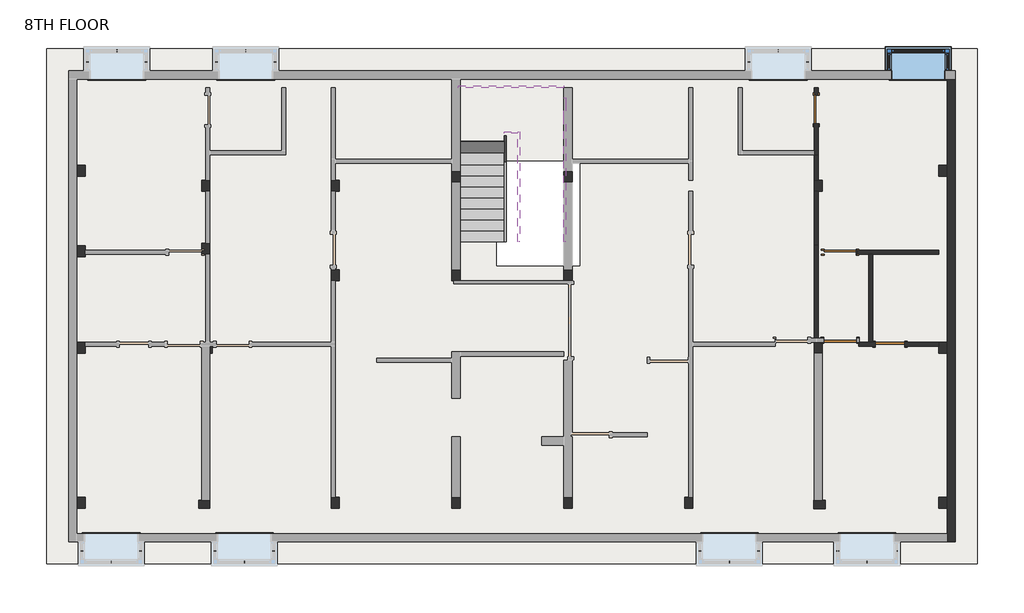
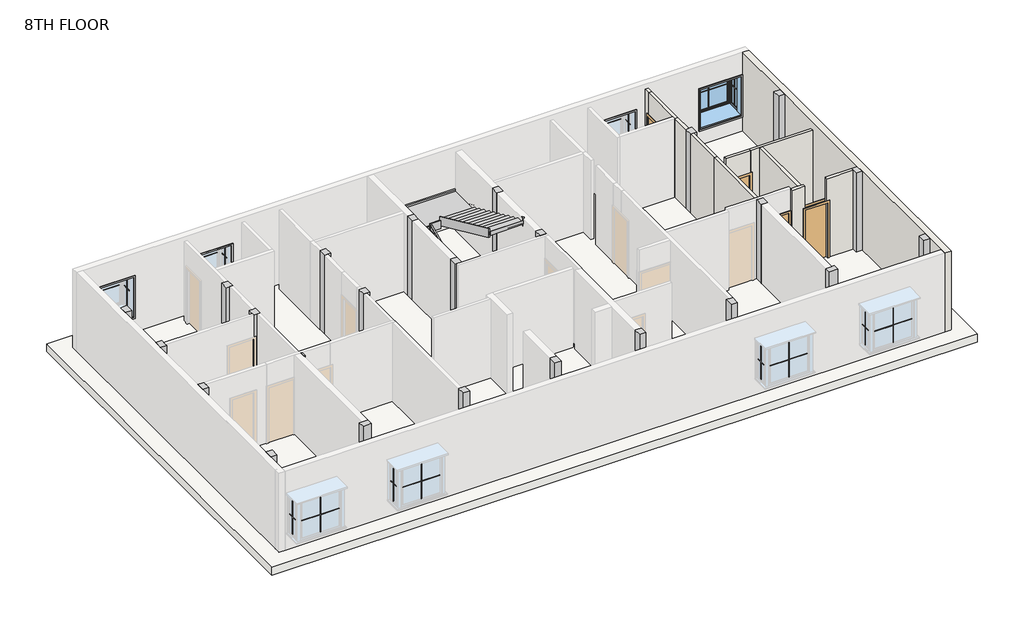
# One storey, part 2 of 2: 32 proxies, 24 columns, 11 walls, 6 members, 4 doors, 1 slab, 1 stair flight, 1 window.
"""IFC4 building model written with IfcOpenShell, lengths in millimetres."""

from ifc_helpers import new_model, si_unit, frame, origin, place, context, project, spatial, polyline, outline, extrude, faceted_brep, transform, mapped, element, save
from components import m_muntin_pattern_2x2_m_muntin_pattern_2x2_c1fd4460, m_muntin_pattern_2x2_m_muntin_pattern_2x2_777b163a, m_trim_window_interior_flat_picture_frame_44e8afef, column_68c8e778, door_1991e9a2, door_a431d384, door_82def9da, m_door_single_panel_3_x7_f8176753, stair_flight_66ca282f, window_19bbd869

model = new_model("IFC4")

# Units and contexts
model_context = context("Model", 3, world=origin())
ifc_project = project(units=[si_unit("LENGTHUNIT", "METRE", prefix="MILLI")], contexts=[model_context])

# Site, building, storey
site = spatial("IfcSite", under=ifc_project)
building = spatial("IfcBuilding", under=site)
storey = spatial("IfcBuildingStorey", under=building, Name="8TH FLOOR", Elevation=28803.6)

# Proxies
placement = place(None, origin())
m_muntin_pattern_2x2_m_muntin_pattern_2x2_shape = m_muntin_pattern_2x2_m_muntin_pattern_2x2_c1fd4460(model_context)
element("IfcBuildingElementProxy", 1, Name="M_Muntin Pattern_2x2 : M_Muntin Pattern_2x2", ObjectType="M_Muntin Pattern_2x2 : M_Muntin Pattern_2x2", at=placement, inside=storey, context=model_context, shape_type="MappedRepresentation", body=[
    mapped(m_muntin_pattern_2x2_m_muntin_pattern_2x2_shape, transform((-11500.7987957, -5499.9182661, 29524.25), x_axis=(-1.0, 0.0, 0.0), y_axis=(0.0, -1.0, 0.0), z_axis=(0.0, 0.0, 1.0))),
])
element("IfcBuildingElementProxy", 2, Name="M_Muntin Pattern_2x2 : M_Muntin Pattern_2x2", ObjectType="M_Muntin Pattern_2x2 : M_Muntin Pattern_2x2", at=placement, inside=storey, context=model_context, shape_type="MappedRepresentation", body=[
    mapped(m_muntin_pattern_2x2_m_muntin_pattern_2x2_shape, transform((-7819.250543, -5499.9182661, 29524.25), x_axis=(-1.0, 0.0, 0.0), y_axis=(0.0, -1.0, 0.0), z_axis=(0.0, 0.0, 1.0))),
])
element("IfcBuildingElementProxy", 3, Name="M_Muntin Pattern_2x2 : M_Muntin Pattern_2x2", ObjectType="M_Muntin Pattern_2x2 : M_Muntin Pattern_2x2", at=placement, inside=storey, context=model_context, shape_type="MappedRepresentation", body=[
    mapped(m_muntin_pattern_2x2_m_muntin_pattern_2x2_shape, transform((5599.7512082, -5499.9182661, 29524.25), x_axis=(-1.0, 0.0, 0.0), y_axis=(0.0, -1.0, 0.0), z_axis=(0.0, 0.0, 1.0))),
])
element("IfcBuildingElementProxy", 4, Name="M_Muntin Pattern_2x2 : M_Muntin Pattern_2x2", ObjectType="M_Muntin Pattern_2x2 : M_Muntin Pattern_2x2", at=placement, inside=storey, context=model_context, shape_type="MappedRepresentation", body=[
    mapped(m_muntin_pattern_2x2_m_muntin_pattern_2x2_shape, transform((9408.6146942, -5499.9182662, 29524.25), x_axis=(-1.0, 0.0, 0.0), y_axis=(0.0, -1.0, 0.0), z_axis=(0.0, 0.0, 1.0))),
])
element("IfcBuildingElementProxy", 5, Name="M_Muntin Pattern_2x2 : M_Muntin Pattern_2x2", ObjectType="M_Muntin Pattern_2x2 : M_Muntin Pattern_2x2", at=placement, inside=storey, context=model_context, shape_type="MappedRepresentation", body=[
    mapped(m_muntin_pattern_2x2_m_muntin_pattern_2x2_shape, transform((-11348.3987957, 8647.7317329, 29524.25), x_axis=(1.0, 0.0, 0.0), y_axis=(0.0, 1.0, 0.0), z_axis=(0.0, 0.0, 1.0))),
])
element("IfcBuildingElementProxy", 6, Name="M_Muntin Pattern_2x2 : M_Muntin Pattern_2x2", ObjectType="M_Muntin Pattern_2x2 : M_Muntin Pattern_2x2", at=placement, inside=storey, context=model_context, shape_type="MappedRepresentation", body=[
    mapped(m_muntin_pattern_2x2_m_muntin_pattern_2x2_shape, transform((-7779.6987993, 8647.7317329, 29524.25), x_axis=(1.0, 0.0, 0.0), y_axis=(0.0, 1.0, 0.0), z_axis=(0.0, 0.0, 1.0))),
])
element("IfcBuildingElementProxy", 7, Name="M_Muntin Pattern_2x2 : M_Muntin Pattern_2x2", ObjectType="M_Muntin Pattern_2x2 : M_Muntin Pattern_2x2", at=placement, inside=storey, context=model_context, shape_type="MappedRepresentation", body=[
    mapped(m_muntin_pattern_2x2_m_muntin_pattern_2x2_shape, transform((6952.301208, 8647.7317329, 29524.25), x_axis=(1.0, 0.0, 0.0), y_axis=(0.0, 1.0, 0.0), z_axis=(0.0, 0.0, 1.0))),
])
element("IfcBuildingElementProxy", 8, Name="M_Muntin Pattern_2x2 : M_Muntin Pattern_2x2", ObjectType="M_Muntin Pattern_2x2 : M_Muntin Pattern_2x2", at=placement, inside=storey, context=model_context, shape_type="MappedRepresentation", body=[
    mapped(m_muntin_pattern_2x2_m_muntin_pattern_2x2_shape, transform((10825.8012075, 8647.7317329, 29524.25), x_axis=(1.0, 0.0, 0.0), y_axis=(0.0, 1.0, 0.0), z_axis=(0.0, 0.0, 1.0))),
])
m_muntin_pattern_2x2_m_muntin_pattern_2x2_2_shape = m_muntin_pattern_2x2_m_muntin_pattern_2x2_777b163a(model_context)
element("IfcBuildingElementProxy", 9, Name="M_Muntin Pattern_2x2 : M_Muntin Pattern_2x2", ObjectType="M_Muntin Pattern_2x2 : M_Muntin Pattern_2x2", at=placement, inside=storey, context=model_context, shape_type="MappedRepresentation", body=[
    mapped(m_muntin_pattern_2x2_m_muntin_pattern_2x2_2_shape, transform((-10690.4737957, -5190.3932661, 29524.25), x_axis=(0.0, 1.0, 0.0), y_axis=(-1.0, 0.0, 0.0), z_axis=(0.0, 0.0, 1.0))),
])
element("IfcBuildingElementProxy", 10, Name="M_Muntin Pattern_2x2 : M_Muntin Pattern_2x2", ObjectType="M_Muntin Pattern_2x2 : M_Muntin Pattern_2x2", at=placement, inside=storey, context=model_context, shape_type="MappedRepresentation", body=[
    mapped(m_muntin_pattern_2x2_m_muntin_pattern_2x2_2_shape, transform((-12311.1237957, -5190.3932661, 29524.25), x_axis=(0.0, -1.0, 0.0), y_axis=(1.0, 0.0, 0.0), z_axis=(0.0, 0.0, 1.0))),
])
element("IfcBuildingElementProxy", 11, Name="M_Muntin Pattern_2x2 : M_Muntin Pattern_2x2", ObjectType="M_Muntin Pattern_2x2 : M_Muntin Pattern_2x2", at=placement, inside=storey, context=model_context, shape_type="MappedRepresentation", body=[
    mapped(m_muntin_pattern_2x2_m_muntin_pattern_2x2_2_shape, transform((-7008.925543, -5190.3932661, 29524.25), x_axis=(0.0, 1.0, 0.0), y_axis=(-1.0, 0.0, 0.0), z_axis=(0.0, 0.0, 1.0))),
])
element("IfcBuildingElementProxy", 12, Name="M_Muntin Pattern_2x2 : M_Muntin Pattern_2x2", ObjectType="M_Muntin Pattern_2x2 : M_Muntin Pattern_2x2", at=placement, inside=storey, context=model_context, shape_type="MappedRepresentation", body=[
    mapped(m_muntin_pattern_2x2_m_muntin_pattern_2x2_2_shape, transform((-8629.575543, -5190.3932661, 29524.25), x_axis=(0.0, -1.0, 0.0), y_axis=(1.0, 0.0, 0.0), z_axis=(0.0, 0.0, 1.0))),
])
element("IfcBuildingElementProxy", 13, Name="M_Muntin Pattern_2x2 : M_Muntin Pattern_2x2", ObjectType="M_Muntin Pattern_2x2 : M_Muntin Pattern_2x2", at=placement, inside=storey, context=model_context, shape_type="MappedRepresentation", body=[
    mapped(m_muntin_pattern_2x2_m_muntin_pattern_2x2_2_shape, transform((6410.0762082, -5190.3932661, 29524.25), x_axis=(0.0, 1.0, 0.0), y_axis=(-1.0, 0.0, 0.0), z_axis=(0.0, 0.0, 1.0))),
])
element("IfcBuildingElementProxy", 14, Name="M_Muntin Pattern_2x2 : M_Muntin Pattern_2x2", ObjectType="M_Muntin Pattern_2x2 : M_Muntin Pattern_2x2", at=placement, inside=storey, context=model_context, shape_type="MappedRepresentation", body=[
    mapped(m_muntin_pattern_2x2_m_muntin_pattern_2x2_2_shape, transform((4789.4262082, -5190.3932661, 29524.25), x_axis=(0.0, -1.0, 0.0), y_axis=(1.0, 0.0, 0.0), z_axis=(0.0, 0.0, 1.0))),
])
element("IfcBuildingElementProxy", 15, Name="M_Muntin Pattern_2x2 : M_Muntin Pattern_2x2", ObjectType="M_Muntin Pattern_2x2 : M_Muntin Pattern_2x2", at=placement, inside=storey, context=model_context, shape_type="MappedRepresentation", body=[
    mapped(m_muntin_pattern_2x2_m_muntin_pattern_2x2_2_shape, transform((10218.9396942, -5190.3932662, 29524.25), x_axis=(0.0, 1.0, 0.0), y_axis=(-1.0, 0.0, 0.0), z_axis=(0.0, 0.0, 1.0))),
])
element("IfcBuildingElementProxy", 16, Name="M_Muntin Pattern_2x2 : M_Muntin Pattern_2x2", ObjectType="M_Muntin Pattern_2x2 : M_Muntin Pattern_2x2", at=placement, inside=storey, context=model_context, shape_type="MappedRepresentation", body=[
    mapped(m_muntin_pattern_2x2_m_muntin_pattern_2x2_2_shape, transform((8598.2896942, -5190.3932661, 29524.25), x_axis=(0.0, -1.0, 0.0), y_axis=(1.0, 0.0, 0.0), z_axis=(0.0, 0.0, 1.0))),
])
element("IfcBuildingElementProxy", 17, Name="M_Muntin Pattern_2x2 : M_Muntin Pattern_2x2", ObjectType="M_Muntin Pattern_2x2 : M_Muntin Pattern_2x2", at=placement, inside=storey, context=model_context, shape_type="MappedRepresentation", body=[
    mapped(m_muntin_pattern_2x2_m_muntin_pattern_2x2_2_shape, transform((-12158.7237957, 8338.2067329, 29524.25), x_axis=(0.0, -1.0, 0.0), y_axis=(1.0, 0.0, 0.0), z_axis=(0.0, 0.0, 1.0))),
])
element("IfcBuildingElementProxy", 18, Name="M_Muntin Pattern_2x2 : M_Muntin Pattern_2x2", ObjectType="M_Muntin Pattern_2x2 : M_Muntin Pattern_2x2", at=placement, inside=storey, context=model_context, shape_type="MappedRepresentation", body=[
    mapped(m_muntin_pattern_2x2_m_muntin_pattern_2x2_2_shape, transform((-10538.0737957, 8338.2067329, 29524.25), x_axis=(0.0, 1.0, 0.0), y_axis=(-1.0, 0.0, 0.0), z_axis=(0.0, 0.0, 1.0))),
])
element("IfcBuildingElementProxy", 19, Name="M_Muntin Pattern_2x2 : M_Muntin Pattern_2x2", ObjectType="M_Muntin Pattern_2x2 : M_Muntin Pattern_2x2", at=placement, inside=storey, context=model_context, shape_type="MappedRepresentation", body=[
    mapped(m_muntin_pattern_2x2_m_muntin_pattern_2x2_2_shape, transform((-8590.0237993, 8338.2067329, 29524.25), x_axis=(0.0, -1.0, 0.0), y_axis=(1.0, 0.0, 0.0), z_axis=(0.0, 0.0, 1.0))),
])
element("IfcBuildingElementProxy", 20, Name="M_Muntin Pattern_2x2 : M_Muntin Pattern_2x2", ObjectType="M_Muntin Pattern_2x2 : M_Muntin Pattern_2x2", at=placement, inside=storey, context=model_context, shape_type="MappedRepresentation", body=[
    mapped(m_muntin_pattern_2x2_m_muntin_pattern_2x2_2_shape, transform((-6969.3737993, 8338.2067329, 29524.25), x_axis=(0.0, 1.0, 0.0), y_axis=(-1.0, 0.0, 0.0), z_axis=(0.0, 0.0, 1.0))),
])
element("IfcBuildingElementProxy", 21, Name="M_Muntin Pattern_2x2 : M_Muntin Pattern_2x2", ObjectType="M_Muntin Pattern_2x2 : M_Muntin Pattern_2x2", at=placement, inside=storey, context=model_context, shape_type="MappedRepresentation", body=[
    mapped(m_muntin_pattern_2x2_m_muntin_pattern_2x2_2_shape, transform((6141.976208, 8338.2067329, 29524.25), x_axis=(0.0, -1.0, 0.0), y_axis=(1.0, 0.0, 0.0), z_axis=(0.0, 0.0, 1.0))),
])
element("IfcBuildingElementProxy", 22, Name="M_Muntin Pattern_2x2 : M_Muntin Pattern_2x2", ObjectType="M_Muntin Pattern_2x2 : M_Muntin Pattern_2x2", at=placement, inside=storey, context=model_context, shape_type="MappedRepresentation", body=[
    mapped(m_muntin_pattern_2x2_m_muntin_pattern_2x2_2_shape, transform((7762.626208, 8338.2067329, 29524.25), x_axis=(0.0, 1.0, 0.0), y_axis=(-1.0, 0.0, 0.0), z_axis=(0.0, 0.0, 1.0))),
])
element("IfcBuildingElementProxy", 23, Name="M_Muntin Pattern_2x2 : M_Muntin Pattern_2x2", ObjectType="M_Muntin Pattern_2x2 : M_Muntin Pattern_2x2", at=placement, inside=storey, context=model_context, shape_type="MappedRepresentation", body=[
    mapped(m_muntin_pattern_2x2_m_muntin_pattern_2x2_2_shape, transform((10015.4762075, 8338.2067329, 29524.25), x_axis=(0.0, -1.0, 0.0), y_axis=(1.0, 0.0, 0.0), z_axis=(0.0, 0.0, 1.0))),
])
element("IfcBuildingElementProxy", 24, Name="M_Muntin Pattern_2x2 : M_Muntin Pattern_2x2", ObjectType="M_Muntin Pattern_2x2 : M_Muntin Pattern_2x2", at=placement, inside=storey, context=model_context, shape_type="MappedRepresentation", body=[
    mapped(m_muntin_pattern_2x2_m_muntin_pattern_2x2_2_shape, transform((11636.1262075, 8338.2067329, 29524.25), x_axis=(0.0, 1.0, 0.0), y_axis=(-1.0, 0.0, 0.0), z_axis=(0.0, 0.0, 1.0))),
])
m_trim_window_interior_flat_picture_frame_shape = m_trim_window_interior_flat_picture_frame_44e8afef(model_context)
element("IfcBuildingElementProxy", 25, Name="M_Trim-Window-Interior-Flat : Picture Frame", ObjectType="M_Trim-Window-Interior-Flat : Picture Frame", at=placement, inside=storey, context=model_context, shape_type="MappedRepresentation", body=[
    mapped(m_trim_window_interior_flat_picture_frame_shape, transform((-11500.7987957, -4712.5932661, 30954.4), x_axis=(-1.0, 0.0, 0.0), y_axis=(0.0, 0.0, 1.0), z_axis=(0.0, 1.0, 0.0))),
])
element("IfcBuildingElementProxy", 26, Name="M_Trim-Window-Interior-Flat : Picture Frame", ObjectType="M_Trim-Window-Interior-Flat : Picture Frame", at=placement, inside=storey, context=model_context, shape_type="MappedRepresentation", body=[
    mapped(m_trim_window_interior_flat_picture_frame_shape, transform((-7819.250543, -4712.5932661, 30954.4), x_axis=(-1.0, 0.0, 0.0), y_axis=(0.0, 0.0, 1.0), z_axis=(0.0, 1.0, 0.0))),
])
element("IfcBuildingElementProxy", 27, Name="M_Trim-Window-Interior-Flat : Picture Frame", ObjectType="M_Trim-Window-Interior-Flat : Picture Frame", at=placement, inside=storey, context=model_context, shape_type="MappedRepresentation", body=[
    mapped(m_trim_window_interior_flat_picture_frame_shape, transform((5599.7512082, -4712.5932661, 30954.4), x_axis=(-1.0, 0.0, 0.0), y_axis=(0.0, 0.0, 1.0), z_axis=(0.0, 1.0, 0.0))),
])
element("IfcBuildingElementProxy", 28, Name="M_Trim-Window-Interior-Flat : Picture Frame", ObjectType="M_Trim-Window-Interior-Flat : Picture Frame", at=placement, inside=storey, context=model_context, shape_type="MappedRepresentation", body=[
    mapped(m_trim_window_interior_flat_picture_frame_shape, transform((9408.6146942, -4712.5932661, 30954.4), x_axis=(-1.0, 0.0, 0.0), y_axis=(0.0, 0.0, 1.0), z_axis=(0.0, 1.0, 0.0))),
])
element("IfcBuildingElementProxy", 29, Name="M_Trim-Window-Interior-Flat : Picture Frame", ObjectType="M_Trim-Window-Interior-Flat : Picture Frame", at=placement, inside=storey, context=model_context, shape_type="MappedRepresentation", body=[
    mapped(m_trim_window_interior_flat_picture_frame_shape, transform((-11348.3987957, 7860.4067329, 30954.4), x_axis=(1.0, 0.0, 0.0), y_axis=(0.0, 0.0, 1.0), z_axis=(0.0, -1.0, 0.0))),
])
element("IfcBuildingElementProxy", 30, Name="M_Trim-Window-Interior-Flat : Picture Frame", ObjectType="M_Trim-Window-Interior-Flat : Picture Frame", at=placement, inside=storey, context=model_context, shape_type="MappedRepresentation", body=[
    mapped(m_trim_window_interior_flat_picture_frame_shape, transform((-7779.6987993, 7860.4067329, 30954.4), x_axis=(1.0, 0.0, 0.0), y_axis=(0.0, 0.0, 1.0), z_axis=(0.0, -1.0, 0.0))),
])
element("IfcBuildingElementProxy", 31, Name="M_Trim-Window-Interior-Flat : Picture Frame", ObjectType="M_Trim-Window-Interior-Flat : Picture Frame", at=placement, inside=storey, context=model_context, shape_type="MappedRepresentation", body=[
    mapped(m_trim_window_interior_flat_picture_frame_shape, transform((6952.301208, 7860.4067329, 30954.4), x_axis=(1.0, 0.0, 0.0), y_axis=(0.0, 0.0, 1.0), z_axis=(0.0, -1.0, 0.0))),
])
element("IfcBuildingElementProxy", 32, Name="M_Trim-Window-Interior-Flat : Picture Frame", ObjectType="M_Trim-Window-Interior-Flat : Picture Frame", at=placement, inside=storey, context=model_context, shape_type="MappedRepresentation", body=[
    mapped(m_trim_window_interior_flat_picture_frame_shape, transform((10825.8012075, 7860.4067329, 30954.4), x_axis=(1.0, 0.0, 0.0), y_axis=(0.0, 0.0, 1.0), z_axis=(0.0, -1.0, 0.0))),
])

# Columns
element("IfcColumn", 33, ObjectType="Rectangular Column : 1'X 9\"", at=placement, inside=storey, context=model_context, shape_type="SweptSolid", body=[
    extrude(outline(polyline([(-12224.6987957, -3709.2932671), (-12224.6987957, -4014.0932671), (-12453.2987957, -4014.0932671), (-12453.2987957, -3709.2932671), (-12224.6987957, -3709.2932671)])), frame((0.0, 0.0, 28803.6), z_axis=(0.0, 0.0, 1.0), x_axis=(1.0, 0.0, 0.0)), (0.0, 0.0, 1.0), 3048.0),
])
element("IfcColumn", 34, ObjectType="Rectangular Column : 1'X 9\"", at=placement, inside=storey, context=model_context, shape_type="SweptSolid", body=[
    extrude(outline(polyline([(-12224.6987957, 583.3067334), (-12224.6987957, 278.5067334), (-12453.2987957, 278.5067334), (-12453.2987957, 583.3067334), (-12224.6987957, 583.3067334)])), frame((0.0, 0.0, 28803.6), z_axis=(0.0, 0.0, 1.0), x_axis=(1.0, 0.0, 0.0)), (0.0, 0.0, 1.0), 3048.0),
])
element("IfcColumn", 35, ObjectType="Rectangular Column : 1'X 9\"", at=placement, inside=storey, context=model_context, shape_type="SweptSolid", body=[
    extrude(outline(polyline([(-12224.6987957, 3256.6567332), (-12224.6987957, 2951.8567332), (-12453.2987957, 2951.8567332), (-12453.2987957, 3256.6567332), (-12224.6987957, 3256.6567332)])), frame((0.0, 0.0, 28803.6), z_axis=(0.0, 0.0, 1.0), x_axis=(1.0, 0.0, 0.0)), (0.0, 0.0, 1.0), 3048.0),
])
element("IfcColumn", 36, ObjectType="Rectangular Column : 1'X 9\"", at=placement, inside=storey, context=model_context, shape_type="Brep", body=[
    faceted_brep([(-8770.2987992, 5066.406733, 28803.6), (-8770.2987992, 4761.606733, 28803.6), (-8884.5987992, 4761.606733, 28803.6), (-8998.8987992, 4761.606733, 28803.6), (-8998.8987992, 5066.406733, 28803.6), (-8884.5987992, 5066.406733, 28803.6), (-8770.2987992, 5066.406733, 31851.6), (-8770.2987992, 4761.606733, 31851.6), (-8884.5987992, 4761.606733, 31851.6), (-8998.8987992, 4761.606733, 31851.6), (-8998.8987992, 5066.406733, 31851.6), (-8884.5987992, 5066.406733, 31851.6)], [[[0, 1, 2, 3, 4, 5]], [[6, 7, 1, 0]], [[7, 8, 9, 3, 2, 1]], [[9, 10, 4, 3]], [[10, 11, 6, 0, 5, 4]], [[6, 11, 10, 9, 8, 7]]]),
])
element("IfcColumn", 37, ObjectType="Rectangular Column : 1'X 9\"", at=placement, inside=storey, context=model_context, shape_type="Brep", body=[
    faceted_brep([(-8770.2987992, 3326.5067332, 28803.6), (-8770.2987992, 3021.7067332, 28803.6), (-8884.598796, 3021.7067332, 28803.6), (-8998.8987992, 3021.7067332, 28803.6), (-8998.8987992, 3326.5067332, 28803.6), (-8884.5987992, 3326.5067332, 28803.6), (-8770.2987992, 3326.5067332, 31851.6), (-8770.2987992, 3021.7067332, 31851.6), (-8884.598796, 3021.7067332, 31851.6), (-8998.8987992, 3021.7067332, 31851.6), (-8998.8987992, 3326.5067332, 31851.6), (-8884.5987992, 3326.5067332, 31851.6)], [[[0, 1, 2, 3, 4, 5]], [[6, 7, 1, 0]], [[7, 8, 9, 3, 2, 1]], [[9, 10, 4, 3]], [[10, 11, 6, 0, 5, 4]], [[6, 11, 10, 9, 8, 7]]]),
])
element("IfcColumn", 38, ObjectType="Rectangular Column : 1'X 9\"", at=placement, inside=storey, context=model_context, shape_type="SweptSolid", body=[
    extrude(outline(polyline([(-8713.148796, 278.5067334), (-8771.750543, 278.5067334), (-8771.750543, 469.0067334), (-8713.148796, 469.0067334), (-8713.148796, 278.5067334)])), frame((0.0, 0.0, 28803.6), z_axis=(0.0, 0.0, 1.0), x_axis=(1.0, 0.0, 0.0)), (0.0, 0.0, 1.0), 3048.0),
])
element("IfcColumn", 39, ObjectType="Rectangular Column : 1'X 9\"", at=placement, inside=storey, context=model_context, shape_type="Brep", body=[
    faceted_brep([(-5188.8987995, 5066.406733, 28803.6), (-5188.8987995, 4761.606733, 28803.6), (-5303.1987995, 4761.606733, 28803.6), (-5417.4987995, 4761.606733, 28803.6), (-5417.4987995, 5066.406733, 28803.6), (-5303.1987995, 5066.406733, 28803.6), (-5188.8987995, 5066.406733, 31851.6), (-5188.8987995, 4761.606733, 31851.6), (-5303.1987995, 4761.606733, 31851.6), (-5417.4987995, 4761.606733, 31851.6), (-5417.4987995, 5066.406733, 31851.6), (-5303.1987995, 5066.406733, 31851.6)], [[[0, 1, 2, 3, 4, 5]], [[6, 7, 1, 0]], [[7, 8, 9, 3, 2, 1]], [[9, 10, 4, 3]], [[10, 11, 6, 0, 5, 4]], [[6, 11, 10, 9, 8, 7]]]),
])
element("IfcColumn", 40, ObjectType="Rectangular Column : 1'X 9\"", at=placement, inside=storey, context=model_context, shape_type="Brep", body=[
    faceted_brep([(-5188.8987995, 2589.9067802, 28803.6), (-5188.8987995, 2285.1067802, 28803.6), (-5303.1987995, 2285.1067802, 28803.6), (-5417.4987995, 2285.1067802, 28803.6), (-5417.4987995, 2589.9067802, 28803.6), (-5303.1987995, 2589.9067802, 28803.6), (-5188.8987995, 2589.9067802, 31851.6), (-5188.8987995, 2285.1067802, 31851.6), (-5303.1987995, 2285.1067802, 31851.6), (-5417.4987995, 2285.1067802, 31851.6), (-5417.4987995, 2589.9067802, 31851.6), (-5303.1987995, 2589.9067802, 31851.6)], [[[0, 1, 2, 3, 4, 5]], [[6, 7, 1, 0]], [[7, 8, 9, 3, 2, 1]], [[9, 10, 4, 3]], [[10, 11, 6, 0, 5, 4]], [[6, 11, 10, 9, 8, 7]]]),
])
element("IfcColumn", 41, ObjectType="Rectangular Column : 1'X 9\"", at=placement, inside=storey, context=model_context, shape_type="Brep", body=[
    faceted_brep([(-5188.8987963, -3709.2932193, 28803.6), (-5188.8987963, -4014.0932193, 28803.6), (-5417.4987963, -4014.0932193, 28803.6), (-5417.4987963, -3709.2932193, 28803.6), (-5303.1987995, -3709.2932193, 28803.6), (-5188.8987963, -3709.2932193, 31851.6), (-5188.8987963, -4014.0932193, 31851.6), (-5417.4987963, -4014.0932193, 31851.6), (-5417.4987963, -3709.2932193, 31851.6), (-5303.1987995, -3709.2932193, 31851.6)], [[[0, 1, 2, 3, 4]], [[5, 6, 1, 0]], [[6, 7, 2, 1]], [[7, 8, 3, 2]], [[8, 9, 5, 0, 4, 3]], [[5, 9, 8, 7, 6]]]),
])
element("IfcColumn", 42, ObjectType="Rectangular Column : 1'X 9\"", at=placement, inside=storey, context=model_context, shape_type="SweptSolid", body=[
    extrude(outline(polyline([(1250.0012085, -3709.2932193), (1250.0012085, -4014.0932193), (1021.4012085, -4014.0932193), (1021.4012085, -3709.2932193), (1250.0012085, -3709.2932193)])), frame((0.0, 0.0, 28803.6), z_axis=(0.0, 0.0, 1.0), x_axis=(1.0, 0.0, 0.0)), (0.0, 0.0, 1.0), 3048.0),
])
element("IfcColumn", 43, ObjectType="Rectangular Column : 1'X 9\"", at=placement, inside=storey, context=model_context, shape_type="Brep", body=[
    faceted_brep([(4590.1012082, -3709.2932193, 28803.6), (4590.1012082, -4014.0932193, 28803.6), (4361.5012082, -4014.0932193, 28803.6), (4361.5012082, -3709.2932193, 28803.6), (4475.8012082, -3709.2932193, 28803.6), (4590.1012082, -3709.2932193, 31851.6), (4590.1012082, -4014.0932193, 31851.6), (4361.5012082, -4014.0932193, 31851.6), (4361.5012082, -3709.2932193, 31851.6), (4475.8012082, -3709.2932193, 31851.6)], [[[0, 1, 2, 3, 4]], [[5, 6, 1, 0]], [[6, 7, 2, 1]], [[7, 8, 3, 2]], [[8, 9, 5, 0, 4, 3]], [[5, 9, 8, 7, 6]]]),
])
element("IfcColumn", 44, ObjectType="Rectangular Column : 1'X 9\"", at=placement, inside=storey, context=model_context, shape_type="SweptSolid", body=[
    extrude(outline(polyline([(11625.9012075, -3709.2932671), (11625.9012075, -4014.0932671), (11397.3012075, -4014.0932671), (11397.3012075, -3709.2932671), (11625.9012075, -3709.2932671)])), frame((0.0, 0.0, 28803.6), z_axis=(0.0, 0.0, 1.0), x_axis=(1.0, 0.0, 0.0)), (0.0, 0.0, 1.0), 3048.0),
])
element("IfcColumn", 45, ObjectType="Rectangular Column : 1'X 9\"", at=placement, inside=storey, context=model_context, shape_type="Brep", body=[
    faceted_brep([(11625.9012075, 583.3067295, 28803.6), (11625.9012075, 278.5067295, 28803.6), (11397.3012075, 278.5067295, 28803.6), (11397.3012075, 469.0067295, 28803.6), (11397.3012075, 583.3067295, 28803.6), (11625.9012075, 583.3067295, 31851.6), (11625.9012075, 278.5067295, 31851.6), (11397.3012075, 278.5067295, 31851.6), (11397.3012075, 469.0067295, 31851.6), (11397.3012075, 583.3067295, 31851.6)], [[[0, 1, 2, 3, 4]], [[5, 6, 1, 0]], [[6, 7, 2, 1]], [[7, 8, 9, 4, 3, 2]], [[9, 5, 0, 4]], [[5, 9, 8, 7, 6]]]),
])
element("IfcColumn", 46, ObjectType="Rectangular Column : 1'X 9\"", at=placement, inside=storey, context=model_context, shape_type="SweptSolid", body=[
    extrude(outline(polyline([(11625.9012075, 5479.1567329), (11625.9012075, 5174.3567329), (11397.3012075, 5174.3567329), (11397.3012075, 5479.1567329), (11625.9012075, 5479.1567329)])), frame((0.0, 0.0, 28803.6), z_axis=(0.0, 0.0, 1.0), x_axis=(1.0, 0.0, 0.0)), (0.0, 0.0, 1.0), 3048.0),
])
element("IfcColumn", 47, ObjectType="Rectangular Column : 1'X 9\"", at=placement, inside=storey, context=model_context, shape_type="Brep", body=[
    faceted_brep([(8172.5040565, 5065.4824989, 28803.6), (8172.5040565, 4760.6824989, 28803.6), (8057.2012047, 4760.6824989, 28803.6), (7943.9040565, 4760.6824989, 28803.6), (7943.9040565, 5065.4824989, 28803.6), (8058.2040565, 5065.4824989, 28803.6), (8172.5040565, 5065.4824989, 31851.6), (8172.5040565, 4760.6824989, 31851.6), (8057.2012047, 4760.6824989, 31851.6), (7943.9040565, 4760.6824989, 31851.6), (7943.9040565, 5065.4824989, 31851.6), (8058.2040565, 5065.4824989, 31851.6)], [[[0, 1, 2, 3, 4, 5]], [[6, 7, 1, 0]], [[7, 8, 9, 3, 2, 1]], [[9, 10, 4, 3]], [[10, 11, 6, 0, 5, 4]], [[6, 11, 10, 9, 8, 7]]]),
])
element("IfcColumn", 48, ObjectType="Rectangular Column : 1'X 9\"", at=placement, inside=storey, context=model_context, shape_type="Brep", body=[
    faceted_brep([(8171.5012047, 583.3067334, 28803.6), (8171.5012047, 278.5067334, 28803.6), (7942.9012047, 278.5067334, 28803.6), (7942.9012047, 583.3067334, 28803.6), (8000.0512079, 583.3067334, 28803.6), (8171.5012047, 583.3067334, 31851.6), (8171.5012047, 278.5067334, 31851.6), (7942.9012047, 278.5067334, 31851.6), (7942.9012047, 583.3067334, 31851.6), (8000.0512079, 583.3067334, 31851.6)], [[[0, 1, 2, 3, 4]], [[5, 6, 1, 0]], [[6, 7, 2, 1]], [[7, 8, 3, 2]], [[8, 9, 5, 0, 4, 3]], [[5, 9, 8, 7, 6]]]),
])
element("IfcColumn", 49, ObjectType="Rectangular Column : 1'X 9\"", at=placement, inside=storey, context=model_context, shape_type="Brep", body=[
    faceted_brep([(-9076.550543, -3785.4932196, 28803.6), (-9000.350543, -3785.4932196, 28803.6), (-8771.750543, -3785.4932196, 28803.6), (-8771.750543, -4014.0932196, 28803.6), (-9076.550543, -4014.0932196, 28803.6), (-9076.550543, -3785.4932196, 31851.6), (-9000.350543, -3785.4932196, 31851.6), (-8771.750543, -3785.4932196, 31851.6), (-8771.750543, -4014.0932196, 31851.6), (-9076.550543, -4014.0932196, 31851.6)], [[[0, 1, 2, 3, 4]], [[5, 6, 7, 2, 1, 0]], [[7, 8, 3, 2]], [[8, 9, 4, 3]], [[9, 5, 0, 4]], [[5, 9, 8, 7, 6]]]),
])
element("IfcColumn", 50, ObjectType="Rectangular Column : 1'X 9\"", at=placement, inside=storey, context=model_context, shape_type="SweptSolid", body=[
    extrude(outline(polyline([(-12453.2987957, 5174.3567339), (-12453.2987957, 5479.1567339), (-12224.6987957, 5479.1567339), (-12224.6987957, 5174.3567339), (-12453.2987957, 5174.3567339)])), frame((0.0, 0.0, 28803.6), z_axis=(0.0, 0.0, 1.0), x_axis=(1.0, 0.0, 0.0)), (0.0, 0.0, 1.0), 3048.0),
])
element("IfcColumn", 51, ObjectType="Rectangular Column : 1'X 9\"", at=placement, inside=storey, context=model_context, shape_type="SweptSolid", body=[
    extrude(outline(polyline([(-1845.5417538, 5320.4067329), (-1845.5417538, 5015.6067329), (-2074.1417538, 5015.6067329), (-2074.1417538, 5320.4067329), (-1845.5417538, 5320.4067329)])), frame((0.0, 0.0, 28803.6), z_axis=(0.0, 0.0, 1.0), x_axis=(1.0, 0.0, 0.0)), (0.0, 0.0, 1.0), 3048.0),
])
element("IfcColumn", 52, ObjectType="Rectangular Column : 1'X 9\"", at=placement, inside=storey, context=model_context, shape_type="SweptSolid", body=[
    extrude(outline(polyline([(1250.0012085, 5320.4067329), (1250.0012085, 5015.6067329), (1021.4012085, 5015.6067329), (1021.4012085, 5320.4067329), (1250.0012085, 5320.4067329)])), frame((0.0, 0.0, 28803.6), z_axis=(0.0, 0.0, 1.0), x_axis=(1.0, 0.0, 0.0)), (0.0, 0.0, 1.0), 3048.0),
])
element("IfcColumn", 53, ObjectType="Rectangular Column : 1'X 9\"", at=placement, inside=storey, context=model_context, shape_type="Brep", body=[
    faceted_brep([(-1845.5417538, 2589.906774, 28803.6), (-1845.5417538, 2285.106774, 28803.6), (-2020.2487998, 2285.106774, 28803.6), (-2074.1417538, 2285.106774, 28803.6), (-2074.1417538, 2589.906774, 28803.6), (-1845.5417538, 2589.906774, 31851.6), (-1845.5417538, 2285.106774, 31851.6), (-2020.2487998, 2285.106774, 31851.6), (-2074.1417538, 2285.106774, 31851.6), (-2074.1417538, 2589.906774, 31851.6)], [[[0, 1, 2, 3, 4]], [[5, 6, 1, 0]], [[6, 7, 8, 3, 2, 1]], [[8, 9, 4, 3]], [[9, 5, 0, 4]], [[5, 9, 8, 7, 6]]]),
])
element("IfcColumn", 54, ObjectType="Rectangular Column : 1'X 9\"", at=placement, inside=storey, context=model_context, shape_type="Brep", body=[
    faceted_brep([(1253.2582462, 2589.9067742, 28803.6), (1253.2582462, 2285.1067742, 28803.6), (1024.6582462, 2285.1067742, 28803.6), (1024.6582462, 2589.9067742, 28803.6), (1250.0012085, 2589.9067742, 28803.6), (1253.2582462, 2589.9067742, 31851.6), (1253.2582462, 2285.1067742, 31851.6), (1024.6582462, 2285.1067742, 31851.6), (1024.6582462, 2589.9067742, 31851.6), (1250.0012085, 2589.9067742, 31851.6)], [[[0, 1, 2, 3, 4]], [[5, 6, 1, 0]], [[6, 7, 2, 1]], [[7, 8, 3, 2]], [[8, 9, 5, 0, 4, 3]], [[5, 9, 8, 7, 6]]]),
])
element("IfcColumn", 55, ObjectType="Rectangular Column : 1'X 9\"", at=placement, inside=storey, context=model_context, shape_type="SweptSolid", body=[
    extrude(outline(polyline([(-1848.7987998, -3709.2932663), (-1848.7987998, -4014.0932663), (-2077.3987998, -4014.0932663), (-2077.3987998, -3709.2932663), (-1848.7987998, -3709.2932663)])), frame((0.0, 0.0, 28803.6), z_axis=(0.0, 0.0, 1.0), x_axis=(1.0, 0.0, 0.0)), (0.0, 0.0, 1.0), 3048.0),
])
column_shape = column_68c8e778(model_context)
element("IfcColumn", 56, ObjectType="Rectangular Column : 1'X 9\"", at=placement, inside=storey, context=model_context, shape_type="MappedRepresentation", body=[
    mapped(column_shape, transform((8094.1646942, -3901.6914801, 0.0), x_axis=(0.0, 1.0, 0.0), y_axis=(-1.0, 0.0, 0.0), z_axis=(0.0, 0.0, 1.0))),
])

# Doors
door_shape = door_1991e9a2(model_context)
element("IfcDoor", 57, ObjectType="M_Door-Single-Panel : 2'11\"X7' 3", at=placement, inside=storey, context=model_context, shape_type="MappedRepresentation", body=[
    mapped(door_shape, transform((8664.274939, 3078.8567332, 28803.6), x_axis=(-1.0, 0.0, 0.0), y_axis=(0.0, -1.0, 0.0), z_axis=(0.0, 0.0, 1.0))),
])
door_2_shape = door_a431d384(model_context)
element("IfcDoor", 58, ObjectType="M_Door-Single-Panel : 2'7\"X7' 2", at=placement, inside=storey, context=model_context, shape_type="MappedRepresentation", body=[
    mapped(door_2_shape, transform((8000.0512079, 7021.3751452, 28803.6), x_axis=(0.0, 1.0, 0.0), y_axis=(-1.0, 0.0, 0.0), z_axis=(0.0, 0.0, 1.0))),
])
door_3_shape = door_82def9da(model_context)
element("IfcDoor", 59, ObjectType="M_Door-Single-Panel : 2'8\"X7'", at=placement, inside=storey, context=model_context, shape_type="MappedRepresentation", body=[
    mapped(door_3_shape, transform((10046.0486694, 526.1567295, 28803.6), x_axis=(-1.0, 0.0, 0.0), y_axis=(0.0, -1.0, 0.0), z_axis=(0.0, 0.0, 1.0))),
])
m_door_single_panel_3_x7_shape = m_door_single_panel_3_x7_f8176753(model_context)
element("IfcDoor", 60, ObjectType="M_Door-Single-Panel : 3'X7'", at=placement, inside=storey, context=model_context, shape_type="MappedRepresentation", body=[
    mapped(m_door_single_panel_3_x7_shape, transform((8666.8012079, 640.4567334, 28803.6), x_axis=(-1.0, 0.0, 0.0), y_axis=(0.0, -1.0, 0.0), z_axis=(0.0, 0.0, 1.0))),
])

# Members
element("IfcMember", 61, ObjectType="Stringer - 2\" Width", at=placement, inside=storey, context=model_context, shape_type="SweptSolid", body=[
    extrude(outline(polyline([(3364.6067329, 28803.6), (3364.6067329, 29003.4262721), (6445.4289342, 30403.8), (7182.0114168, 30403.8), (3661.5714168, 28803.6), (3364.6067329, 28803.6)])), frame((-1896.3417538, 0.0, 0.0), z_axis=(1.0, 0.0, 0.0), x_axis=(0.0, 1.0, 0.0)), (0.0, 0.0, 1.0), 50.8),
])
element("IfcMember", 62, ObjectType="Stringer - 2\" Width", at=placement, inside=storey, context=model_context, shape_type="SweptSolid", body=[
    extrude(outline(polyline([(-1896.3417538, 7631.8067329), (-1896.3417538, 7682.6067329), (1021.4012085, 7682.6067329), (1021.4012085, 7631.8067329), (-1896.3417538, 7631.8067329)])), frame((0.0, 0.0, 30099.0), z_axis=(0.0, 0.0, 1.0), x_axis=(1.0, 0.0, 0.0)), (0.0, 0.0, 1.0), 304.8),
])
element("IfcMember", 63, ObjectType="Stringer - 2\" Width", at=placement, inside=storey, context=model_context, shape_type="SweptSolid", body=[
    extrude(outline(polyline([(6618.562049, 30099.0), (3364.6067329, 31578.0705982), (3364.6067329, 31912.8808176), (7355.1445316, 30099.0), (6618.562049, 30099.0)])), frame((1021.4012085, 0.0, 0.0), z_axis=(1.0, 0.0, 0.0), x_axis=(0.0, 1.0, 0.0)), (0.0, 0.0, 1.0), 50.8),
])
element("IfcMember", 64, ObjectType="Stringer - 2\" Width", at=placement, inside=storey, context=model_context, shape_type="SweptSolid", body=[
    extrude(outline(polyline([(3364.6067329, 28803.6), (3364.6067329, 29003.4262721), (6361.8067329, 30365.7899085), (6361.8067329, 30030.9796892), (3661.5714168, 28803.6), (3364.6067329, 28803.6)])), frame((-629.5987998, 0.0, 0.0), z_axis=(1.0, 0.0, 0.0), x_axis=(0.0, 1.0, 0.0)), (0.0, 0.0, 1.0), 50.8),
])
element("IfcMember", 65, ObjectType="Stringer - 2\" Width", at=placement, inside=storey, context=model_context, shape_type="SweptSolid", body=[
    extrude(outline(polyline([(-629.5987998, 6361.8067329), (-629.5987998, 6412.6067329), (-248.5987915, 6412.6067329), (-248.5987915, 6361.8067329), (-629.5987998, 6361.8067329)])), frame((0.0, 0.0, 30099.0), z_axis=(0.0, 0.0, 1.0), x_axis=(1.0, 0.0, 0.0)), (0.0, 0.0, 1.0), 304.8),
])
element("IfcMember", 66, ObjectType="Stringer - 2\" Width", at=placement, inside=storey, context=model_context, shape_type="SweptSolid", body=[
    extrude(outline(polyline([(6412.6067329, 30527.4262721), (6412.6067329, 30192.6160528), (3364.6067329, 31578.0705982), (3364.6067329, 31912.8808176), (6412.6067329, 30527.4262721)])), frame((-248.5987915, 0.0, 0.0), z_axis=(1.0, 0.0, 0.0), x_axis=(0.0, 1.0, 0.0)), (0.0, 0.0, 1.0), 50.8),
])

# Slab
element("IfcSlab", 67, ObjectType="Generic - 12\"", at=placement, inside=storey, context=model_context, shape_type="SweptSolid", body=[
    extrude(outline(polyline([(12464.1012075, 8698.6067329), (12464.1012075, -5550.7932662), (-13291.4987957, -5550.7932662), (-13291.4987957, 8698.6067329), (12464.1012075, 8698.6067329)]), holes=[polyline([(1456.6270108, 2700.0220048), (1456.6270108, 5595.6220048), (-829.3729892, 5595.6220048), (-829.3729892, 2700.0220048), (1456.6270108, 2700.0220048)])]), frame((0.0, 0.0, 28498.8), z_axis=(0.0, 0.0, 1.0), x_axis=(1.0, 0.0, 0.0)), (0.0, 0.0, 1.0), 304.8),
])

# Stair flight
stair_flight_shape = stair_flight_66ca282f(model_context)
element("IfcStairFlight", 68, ObjectType="2\" Tread 1\" Nosing 1/4\" Riser", at=placement, inside=storey, context=model_context, shape_type="MappedRepresentation", body=[
    mapped(stair_flight_shape, transform((0.0, 0.0, 0.0), x_axis=(1.0, 0.0, 0.0), y_axis=(0.0, 1.0, 0.0), z_axis=(0.0, 0.0, 1.0))),
])

# Walls
element("IfcWall", 69, ObjectType="4.5\"", at=placement, inside=storey, context=model_context, shape_type="SweptSolid", body=[
    extrude(outline(polyline([(28803.6, 9131.6486701), (31851.6, 9131.6486701), (31851.6, 8245.174939), (30937.2, 8245.174939), (30937.2, 9108.774939), (28803.6, 9108.774939), (28803.6, 9131.6486701)])), frame((0.0, 3021.7067332, 0.0), z_axis=(0.0, 1.0, 0.0), x_axis=(0.0, 0.0, 1.0)), (0.0, 0.0, 1.0), 114.3),
])
element("IfcWall", 70, ObjectType="4.5\"", at=placement, inside=storey, context=model_context, shape_type="Brep", body=[
    faceted_brep([(7942.9012079, 5764.9067329, 31851.6), (7942.9012079, 5879.2067329, 31851.6), (7942.9012079, 7415.0751452, 31851.6), (7942.9012079, 7415.0751452, 30937.2), (7942.9012079, 6627.6751452, 30937.2), (7942.9012079, 6627.6751452, 28803.6), (7942.9012079, 5879.2067329, 28803.6), (7942.9012079, 5764.9067329, 28803.6), (8057.2012079, 7415.0751452, 31851.6), (8057.2012079, 5764.9067329, 31851.6), (8057.2012079, 5764.9067329, 28803.6), (8057.2012079, 6627.6751452, 28803.6), (8057.2012079, 6627.6751452, 30937.2), (8057.2012079, 7415.0751452, 30937.2)], [[[0, 1, 2, 3, 4, 5, 6, 7]], [[8, 9, 10, 11, 12, 13]], [[10, 7, 6, 5, 11]], [[2, 1, 0, 9, 8]], [[2, 8, 13, 3]], [[12, 4, 3, 13]], [[4, 12, 11, 5]], [[0, 7, 10, 9]]]),
])
element("IfcWall", 71, ObjectType="4.5\"", at=placement, inside=storey, context=model_context, shape_type="Brep", body=[
    faceted_brep([(7942.9012079, 7631.8067329, 28803.6), (7942.9012079, 7415.0751452, 28803.6), (7942.9012079, 7415.0751452, 30937.2), (7942.9012079, 7415.0751452, 31851.6), (7942.9012079, 7631.8067329, 31851.6), (8057.2012079, 7631.8067329, 28803.6), (8057.2012079, 7631.8067329, 31851.6), (8057.2012079, 7415.0751452, 31851.6), (8057.2012079, 7415.0751452, 30937.2), (8057.2012079, 7415.0751452, 28803.6)], [[[0, 1, 2, 3, 4]], [[5, 6, 7, 8, 9]], [[1, 0, 5, 9]], [[3, 2, 1, 9, 8, 7]], [[4, 3, 7, 6]], [[0, 4, 6, 5]]]),
])
element("IfcWall", 72, ObjectType="4.5\"", at=placement, inside=storey, context=model_context, shape_type="Brep", body=[
    faceted_brep([(8057.2012047, 3270.1432417, 28803.6), (8057.2012047, 4760.6824989, 28803.6), (8057.2012047, 4760.6824989, 31851.6), (8057.2012047, 3270.1432417, 31851.6), (7942.9012047, 3270.1432417, 28803.6), (7942.9012047, 3270.1432417, 31851.6), (7942.9012047, 4760.6824989, 31851.6), (7942.9012047, 4760.6824989, 28803.6), (7943.9040565, 4760.6824989, 28803.6), (7943.9040565, 4760.6824989, 31851.6)], [[[0, 1, 2, 3]], [[4, 5, 6, 7]], [[1, 0, 4, 7, 8]], [[2, 1, 8, 7, 6, 9]], [[3, 2, 9, 6, 5]], [[0, 3, 5, 4]]]),
])
element("IfcWall", 73, ObjectType="4.5\"", at=placement, inside=storey, context=model_context, shape_type="Brep", body=[
    faceted_brep([(7942.9012079, 3270.1432417, 28803.6), (7942.9012079, 697.6067334, 28803.6), (7942.9012079, 697.6067334, 31851.6), (7942.9012079, 3270.1432417, 31851.6), (8057.2012079, 3270.1432417, 28803.6), (8057.2012079, 3270.1432417, 31851.6), (8057.2012079, 697.6067334, 31851.6), (8057.2012079, 697.6067334, 28803.6), (8000.0512079, 697.6067334, 28803.6), (8000.0512079, 697.6067334, 31851.6)], [[[0, 1, 2, 3]], [[4, 5, 6, 7]], [[1, 0, 4, 7, 8]], [[3, 2, 9, 6, 5]], [[0, 3, 5, 4]], [[2, 1, 8, 7, 6, 9]]]),
])
element("IfcWall", 74, ObjectType="4.5\"", at=placement, inside=storey, context=model_context, shape_type="SweptSolid", body=[
    extrude(outline(polyline([(8058.2040565, 5763.9824989), (8058.2040565, 5065.4824989), (7943.9040565, 5065.4824989), (7943.9040565, 5763.9824989), (8058.2040565, 5763.9824989)])), frame((0.0, 0.0, 28803.6), z_axis=(0.0, 0.0, 1.0), x_axis=(1.0, 0.0, 0.0)), (0.0, 0.0, 1.0), 3048.0),
])
element("IfcWall", 75, ObjectType="4.5\" 2", at=placement, inside=storey, context=model_context, shape_type="Brep", body=[
    faceted_brep([(9182.4486694, 469.0067295, 28803.6), (9639.6486694, 469.0067295, 28803.6), (9639.6486694, 469.0067295, 31851.6), (9182.4486694, 469.0067295, 31851.6), (9182.4486694, 583.3067295, 28803.6), (9182.4486694, 583.3067295, 31851.6), (9451.1098918, 583.3067295, 31851.6), (9565.4098918, 583.3067295, 31851.6), (9639.6486694, 583.3067295, 31851.6), (9639.6486694, 583.3067295, 28803.6), (9565.4098918, 583.3067295, 28803.6), (9451.1098918, 583.3067295, 28803.6)], [[[0, 1, 2, 3]], [[4, 5, 6, 7, 8, 9, 10, 11]], [[1, 0, 4, 11, 10, 9]], [[2, 1, 9, 8]], [[3, 2, 8, 7, 6, 5]], [[0, 3, 5, 4]]]),
])
element("IfcWall", 76, ObjectType="4.5\" 2", at=placement, inside=storey, context=model_context, shape_type="SweptSolid", body=[
    extrude(outline(polyline([(28803.6, 11397.3012075), (31851.6, 11397.3012075), (31851.6, 10443.8236977), (30937.2, 10443.8236977), (30937.2, 10452.4486694), (28803.6, 10452.4486694), (28803.6, 11397.3012075)])), frame((0.0, 469.0067295, 0.0), z_axis=(0.0, 1.0, 0.0), x_axis=(0.0, 0.0, 1.0)), (0.0, 0.0, 1.0), 114.3),
])
element("IfcWall", 77, ObjectType="4.5\" 2", at=placement, inside=storey, context=model_context, shape_type="SweptSolid", body=[
    extrude(outline(polyline([(9565.4098918, 3021.7067332), (9565.4098918, 583.3067295), (9451.1098918, 583.3067295), (9451.1098918, 3021.7067332), (9565.4098918, 3021.7067332)])), frame((0.0, 0.0, 28803.6), z_axis=(0.0, 0.0, 1.0), x_axis=(1.0, 0.0, 0.0)), (0.0, 0.0, 1.0), 3048.0),
])
element("IfcWall", 78, ObjectType="4.5\" 2", at=placement, inside=storey, context=model_context, shape_type="Brep", body=[
    faceted_brep([(9131.6486701, 3021.7067332, 28803.6), (9451.1098918, 3021.7067332, 28803.6), (9565.4098918, 3021.7067332, 28803.6), (11397.3012075, 3021.7067332, 28803.6), (11397.3012075, 3021.7067332, 31851.6), (9565.4098918, 3021.7067332, 31851.6), (9451.1098918, 3021.7067332, 31851.6), (9131.6486701, 3021.7067332, 31851.6), (9131.6486701, 3136.0067332, 28803.6), (9131.6486701, 3136.0067332, 31851.6), (11397.3012075, 3136.0067332, 31851.6), (11397.3012075, 3136.0067332, 28803.6)], [[[0, 1, 2, 3, 4, 5, 6, 7]], [[8, 9, 10, 11]], [[3, 2, 1, 0, 8, 11]], [[4, 3, 11, 10]], [[7, 6, 5, 4, 10, 9]], [[0, 7, 9, 8]]]),
])
element("IfcWall", 79, ObjectType="9\"", at=placement, inside=storey, context=model_context, shape_type="Brep", body=[
    faceted_brep([(11625.9012075, 7860.4067329, 28803.6), (11625.9012075, 5479.1567329, 28803.6), (11625.9012075, 5174.3567329, 28803.6), (11625.9012075, 583.3067295, 28803.6), (11625.9012075, 278.5067295, 28803.6), (11625.9012075, -3709.2932671, 28803.6), (11625.9012075, -4014.0932671, 28803.6), (11625.9012075, -4712.5932662, 28803.6), (11625.9012075, -4941.1932662, 28803.6), (11625.9012075, -4941.1932662, 31851.6), (11625.9012075, -4712.5932662, 31851.6), (11625.9012075, -4014.0932671, 31851.6), (11625.9012075, -3709.2932671, 31851.6), (11625.9012075, 278.5067295, 31851.6), (11625.9012075, 583.3067295, 31851.6), (11625.9012075, 5174.3567329, 31851.6), (11625.9012075, 5479.1567329, 31851.6), (11625.9012075, 7860.4067329, 31851.6), (11854.5012075, 7860.4067329, 28803.6), (11854.5012075, 7860.4067329, 31851.6), (11854.5012075, -4941.1932662, 31851.6), (11854.5012075, -4941.1932662, 28803.6)], [[[0, 1, 2, 3, 4, 5, 6, 7, 8, 9, 10, 11, 12, 13, 14, 15, 16, 17]], [[18, 19, 20, 21]], [[8, 7, 6, 5, 4, 3, 2, 1, 0, 18, 21]], [[17, 16, 15, 14, 13, 12, 11, 10, 9, 20, 19]], [[0, 17, 19, 18]], [[9, 8, 21, 20]]]),
])

# Window
window_shape = window_19bbd869(model_context)
element("IfcWindow", 80, ObjectType="4'.8\"x3'.8\"", at=placement, inside=storey, context=model_context, shape_type="MappedRepresentation", body=[
    mapped(window_shape, transform((10825.8012075, 7974.7067329, 28803.6), x_axis=(1.0, 0.0, 0.0), y_axis=(0.0, 1.0, 0.0), z_axis=(0.0, 0.0, 1.0))),
])

save(model, "model.ifc")

# Revit data of these elements
# Type "M_Muntin Pattern_2x2 : M_Muntin Pattern_2x2"
#   Width [instance default] = 3' - 11.24409"
#   Thickness = 0' - 0 1/2"
#   Height [instance default] = 3' - 11.24409"
#   Distance = 0' - 0 3/4"
#   Interior Material [instance default] = none
#   Exterior Material [instance default] = none
#   Default Elevation = 0
# Type "M_Trim-Window-Interior-Flat : Picture Frame"
#   Trim Thickness_Picture Frame = 0' - 1.1811"
#   Trim Width = 0' - 2.3622"
#   Trim Thickness_with Sill = 0' - 0.7874"
#   Sill Thickness = 0' - 1.1811"
#   Opening Width [instance default] = 1' - 11.62205"
#   Opening Height [instance default] = 2' - 11.43307"
#   Default Elevation = 3' - 11.24409"
#   Sill = no
#   Picture Frame = yes
#   Trim Material [instance default] = none
# Type "Rectangular Column : 1'X 9\""
#   Assembly Code = "B1010200"
#   Depth = 1' - 0"
#   Offset Base = 0' - 0"
#   Offset Top = 0' - 0"
#   Width = 0' - 9"
#   Material = none
# Type "M_Door-Single-Panel : 2'11\"X7' 3"
#   Type Mark = "12"
#   Construction Type Id = "DOOR"
#   Assembly Code = "C1020300"
#   Analytic Construction = "Wooden"
#   Thickness = 0' - 1.9685"
#   Thermal Resistance (R) = 2.5876 (h·ft²·°F)/BTU
#   Swing Angle [instance default] = 90.00°
#   Heat Transfer Coefficient (U) = 0.3865 BTU/(h·ft²·°F)
#   Height = 7' - 0"
#   Trim Projection Ext = 0' - 0.98425"
#   Trim Projection Int = 0' - 0.98425"
#   Trim Width = 0' - 3.14961"
#   Width = 2' - 11"
#   Define Thermal Properties by = 1
#   Panel Material = Wood - Birch - Solid Stained Light Low Gloss
#   Trim Material = Paint - Sienna
#   Visual Light Transmittance = 0
#   Solar Heat Gain Coefficient = 0
#   Function = (empty or 0)
#   Wall Closure = (empty or 0)
# Type "M_Door-Single-Panel : 2'7\"X7' 2"
#   Type Mark = "13"
#   Construction Type Id = "DOOR"
#   Assembly Code = "C1020300"
#   Analytic Construction = "Wooden"
#   Thickness = 0' - 1.9685"
#   Thermal Resistance (R) = 2.5876 (h·ft²·°F)/BTU
#   Swing Angle [instance default] = 90.00°
#   Heat Transfer Coefficient (U) = 0.3865 BTU/(h·ft²·°F)
#   Height = 7' - 0"
#   Trim Projection Ext = 0' - 0.98425"
#   Trim Projection Int = 0' - 0.98425"
#   Trim Width = 0' - 3.14961"
#   Width = 2' - 7"
#   Define Thermal Properties by = 1
#   Panel Material = Wood - Birch - Solid Stained Light Low Gloss
#   Trim Material = Paint - Sienna
#   Visual Light Transmittance = 0
#   Solar Heat Gain Coefficient = 0
#   Function = (empty or 0)
#   Wall Closure = (empty or 0)
# Type "M_Door-Single-Panel : 2'8\"X7'"
#   Type Mark = "9"
#   Construction Type Id = "DOOR"
#   Assembly Code = "C1020300"
#   Analytic Construction = "Wooden"
#   Thickness = 0' - 1.9685"
#   Thermal Resistance (R) = 2.5876 (h·ft²·°F)/BTU
#   Swing Angle [instance default] = 90.00°
#   Heat Transfer Coefficient (U) = 0.3865 BTU/(h·ft²·°F)
#   Height = 7' - 0"
#   Trim Projection Ext = 0' - 0.98425"
#   Trim Projection Int = 0' - 0.98425"
#   Trim Width = 0' - 3.14961"
#   Width = 2' - 8"
#   Define Thermal Properties by = 1
#   Panel Material = Wood - Birch - Solid Stained Light Low Gloss
#   Trim Material = Paint - Sienna
#   Visual Light Transmittance = 0
#   Solar Heat Gain Coefficient = 0
#   Function = (empty or 0)
#   Wall Closure = (empty or 0)
# Type "M_Door-Single-Panel : 3'X7'"
#   Type Mark = "11"
#   Construction Type Id = "DOOR"
#   Assembly Code = "C1020300"
#   Analytic Construction = "Wooden"
#   Thickness = 0' - 1.9685"
#   Thermal Resistance (R) = 2.5876 (h·ft²·°F)/BTU
#   Swing Angle [instance default] = 90.00°
#   Heat Transfer Coefficient (U) = 0.3865 BTU/(h·ft²·°F)
#   Height = 7' - 0"
#   Trim Projection Ext = 0' - 0.98425"
#   Trim Projection Int = 0' - 0.98425"
#   Trim Width = 0' - 3.14961"
#   Width = 3' - 0"
#   Define Thermal Properties by = 1
#   Panel Material = Wood - Birch - Solid Stained Light Low Gloss
#   Trim Material = Paint - Sienna
#   Visual Light Transmittance = 0
#   Solar Heat Gain Coefficient = 0
#   Function = (empty or 0)
#   Wall Closure = (empty or 0)
# Type "Generic - 12\""
#   Assembly Code = "B1010"
#   Function = 0
#   Layers, outside or top first: 1' - 0" no material (function 1)
# Type "4.5\""
#   Assembly Code = "B2010"
#   Layers, outside or top first: 0' - 4 1/2" no material (function 1)
# Type "4.5\" 2"
#   Assembly Code = "B2010"
#   Layers, outside or top first: 0' - 4 1/2" no material (function 1)
# Type "9\""
#   Assembly Code = "B2010"
#   Layers, outside or top first: 0' - 9" no material (function 1)
# Type "4'.8\"x3'.8\""
#   Type Mark = "20"
#   Fire Rating = "0.5h"
#   Assembly Code = "B2020100"
#   Analytic Construction = "1/8 in Pilkington single glazing"
#   Width = 4' - 11.05512"
#   Wall Thickness [instance default] = 0' - 5.90551"
#   Visual Light Transmittance = 0.9
#   Trim Width = 5' - 7.05512"
#   Trim Height = 4' - 11.05512"
#   Thermal Resistance (R) = 1.5394 (h·ft²·°F)/BTU
#   Solar Heat Gain Coefficient = 0.86
#   Rough Width = 4' - 11.64567"
#   Rough Height = 4' - 11.64567"
#   Height 1 = 5' - 1.05512"
#   Height = 4' - 11.05512"
#   Heat Transfer Coefficient (U) = 0.6496 BTU/(h·ft²·°F)
#   Depth = 1' - 11.62205"
#   Default Sill Height = 1' - 11.62205"
#   Side Muntin Visibility = yes
#   Center Muntin Visibility = yes
#   Interior Trim Visibility [instance default] = yes
#   Exterior Trim Visibility [instance default] = yes
#   Side Muntin Pattern = M_Muntin Pattern_2x2 : M_Muntin Pattern_2x2
#   Center Muntin Pattern = M_Muntin Pattern_2x2 : M_Muntin Pattern_2x2
#   Interior Trim Material = Wood - Stained
#   Exterior Trim Material = Clad - White
#   Exterior Trim = element 422966
#   Interior Trim = M_Trim-Window-Interior-Flat : Picture Frame
#   Interior Frame Material = Wood - Stained
#   Glass Panel Material = Glass
#   Exterior Frame Material = Clad - White
#   Wall Closure = (empty or 0)
# Elements 1, 2, 3, 4, 5, 6, 7, 8 (IfcBuildingElementProxy, "M_Muntin Pattern_2x2 : M_Muntin Pattern_2x2")
#   Width = 4' - 5.55512"
#   Height = 4' - 5.55512"
#   Interior Material = Wood - Stained
#   Exterior Material = Clad - White
#   Phase Created = New Construction
#   Materials on its faces: "Clad - White", "Wood - Stained"
# Elements 9, 10, 11, 12, 13, 14, 15, 16, 17, 18, 19, 20, 21, 22, 23, 24 (IfcBuildingElementProxy, "M_Muntin Pattern_2x2 : M_Muntin Pattern_2x2")
#   Width = 1' - 2.12205"
#   Height = 4' - 5.55512"
#   Interior Material = Wood - Stained
#   Exterior Material = Clad - White
#   Phase Created = New Construction
#   Materials on its faces: "Clad - White", "Wood - Stained"
# Elements 25, 26, 27, 28, 29, 30, 31, 32 (IfcBuildingElementProxy, "M_Trim-Window-Interior-Flat : Picture Frame")
#   Opening Width = 4' - 11.05512"
#   Opening Height = 5' - 1.05512"
#   Trim Material = Wood - Stained
#   Phase Created = New Construction
#   Materials on its faces: "Wood - Stained"
# Elements 33, 34, 35, 36, 37, 38, 39, 40, 41, 42, 43, 44, 45, 46, 47, 48, 49, 50, 51, 52, 53, 54, 55 (IfcColumn, "Rectangular Column : 1'X 9\"")
#   Phase Created = New Construction
#   Materials on its faces: "Default Wall"
# Element 56 (IfcColumn, "Rectangular Column : 1'X 9\"")
#   Phase Created = New Construction
# Element 57 (IfcDoor, "M_Door-Single-Panel : 2'11\"X7' 3")
#   Swing Angle = 90.00°
#   Phase Created = New Construction
#   Materials on its faces: "Paint - Sienna", "Wood - Birch - Solid Stained Light Low Gloss"
# Element 58 (IfcDoor, "M_Door-Single-Panel : 2'7\"X7' 2")
#   Swing Angle = 90.00°
#   Phase Created = New Construction
#   Materials on its faces: "Paint - Sienna", "Wood - Birch - Solid Stained Light Low Gloss"
# Element 59 (IfcDoor, "M_Door-Single-Panel : 2'8\"X7'")
#   Swing Angle = 90.00°
#   Phase Created = New Construction
#   Materials on its faces: "Paint - Sienna", "Wood - Birch - Solid Stained Light Low Gloss"
# Element 60 (IfcDoor, "M_Door-Single-Panel : 3'X7'")
#   Swing Angle = 90.00°
#   Phase Created = New Construction
#   Materials on its faces: "Paint - Sienna", "Wood - Birch - Solid Stained Light Low Gloss"
# Elements 61, 62, 63, 64, 65, 66 (IfcMember, "Stringer - 2\" Width")
#   Phase Created = New Construction
# Element 67 (IfcSlab, "Generic - 12\"")
#   Height Offset From Level = 0' - 0"
#   Phase Created = New Construction
#   Materials on its faces: "Default Floor"
# Element 68 (IfcStairFlight, "2\" Tread 1\" Nosing 1/4\" Riser")
#   Phase Created = New Construction
# Elements 69, 70, 71, 72, 73, 74 (IfcWall, "4.5\"")
#   Top Offset = -0' - 6"
#   Base Offset = 0' - 0"
#   wall height = 10' - 0"
#   Phase Created = New Construction
#   Base Constraint = 8TH FLOOR
#   Top Constraint = 9TH FLOOR
#   Materials on its faces: "Default Wall"
# Elements 75, 76, 77, 78 (IfcWall, "4.5\" 2")
#   Top Offset = -0' - 6"
#   Base Offset = 0' - 0"
#   wall height = 10' - 0"
#   Phase Created = New Construction
#   Base Constraint = 8TH FLOOR
#   Top Constraint = 9TH FLOOR
#   Materials on its faces: "Default Wall"
# Element 79 (IfcWall, "9\"")
#   Top Offset = -0' - 6"
#   Base Offset = 0' - 0"
#   wall height = 10' - 0"
#   Phase Created = New Construction
#   Base Constraint = 8TH FLOOR
#   Top Constraint = 9TH FLOOR
#   Materials on its faces: "Default Wall"
# Element 80 (IfcWindow, "4'.8\"x3'.8\"")
#   Mark = "290"
#   Interior Trim Visibility = yes
#   Exterior Trim Visibility = yes
#   Phase Created = New Construction
#   Materials on its faces: "Clad - White", "Wood - Stained", "Glass"
# Materials
#   "Wood - Birch - Solid Stained Light Low Gloss": class "Wood", colour RGB 210 159 95, transparency 0, Cost = 0
#   "Paint - Sienna": colour RGB 118 70 51, transparency 0, Cost = 0
#   "Wood - Stained": class "Wood", colour RGB 224 178 126, transparency 0, Cost = 0
#   "Clad - White": class "Wood", colour RGB 242 242 238, transparency 0, Cost = 0
#   "Glass": class "Glass", colour RGB 0 128 192, transparency 0.75, Description = "Soda Lime Glass", Cost = 0
#   "Default Wall": colour RGB 128 128 128, transparency 0, Cost = 0
#   "Default Floor": colour RGB 128 128 128, transparency 0, Cost = 0
